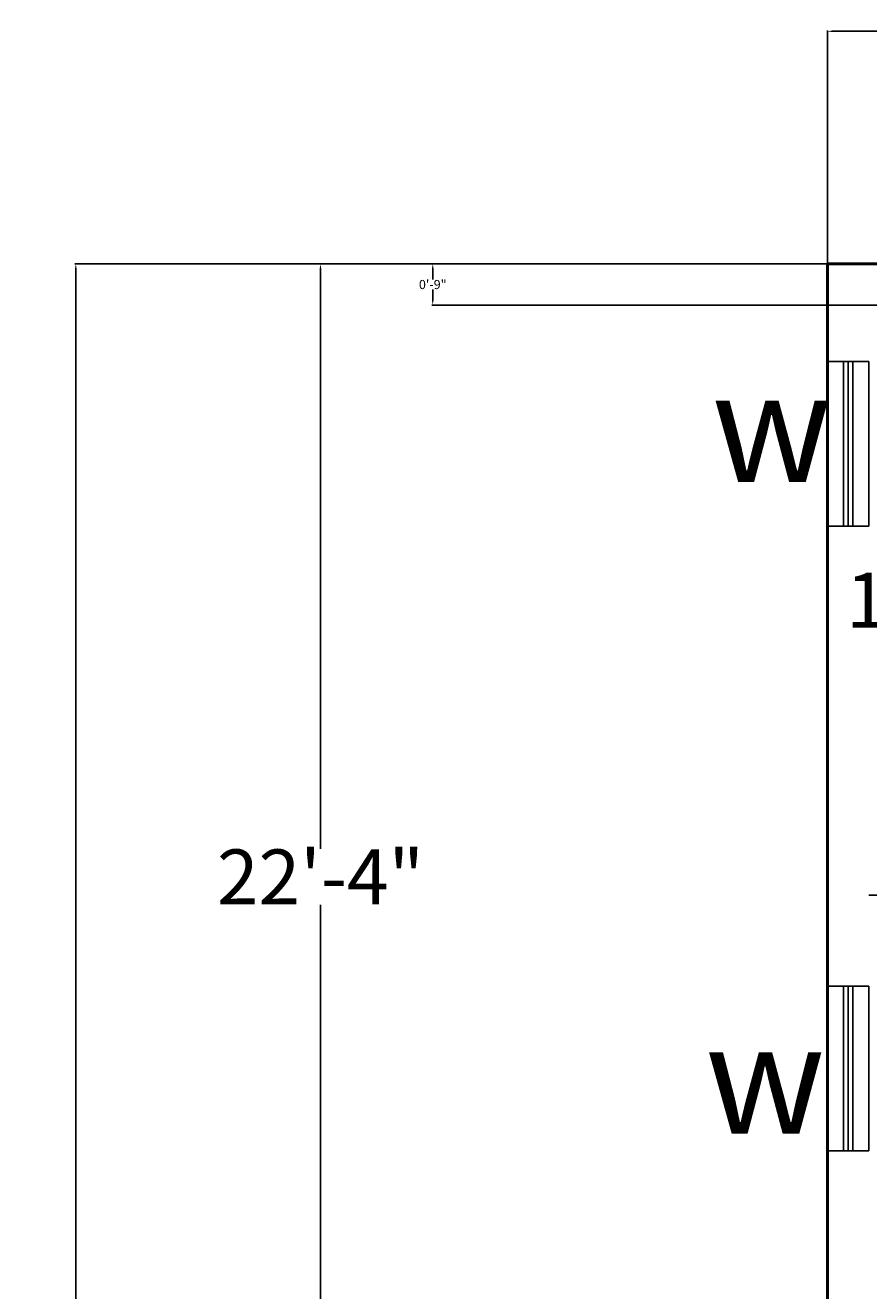
# Model space of a CAD drawing. Units: inches. Extents: x 409 to 7572, y 7 to 725.
# Tile 16 of 38: x 2800 to 2984, y 448 to 725. Entities that reach past the tile are written whole.
import ezdxf

# ---------------------------------------------------------------- set-up
doc = ezdxf.new("R2010")
doc.units = ezdxf.units.IN
doc.header["$MEASUREMENT"] = 0
for name, color, linetype, lineweight in [('A-ANNO-DIMS', 2, 'Continuous', 18), ('A-ANNO-SYMB', 3, 'Continuous', 25), ('A-GLAZ', 4, 'Continuous', 25), ('A-WALL', 7, 'Continuous', 50)]:
    doc.layers.add(name, color=color, linetype=linetype, lineweight=lineweight)
doc.styles.get("Standard").update_dxf_attribs({"font": 'arial.ttf'})
doc.dimstyles.get("Standard").update_dxf_attribs({"dimtxt": 2, "dimasz": 1, "dimexe": 0.18, "dimexo": 0.0625, "dimgap": 0.09, "dimtad": 0, "dimtih": 1, "dimtoh": 1, "dimdec": 0, "dimzin": 0, "dimdsep": 46, "dimlunit": 3, "dimtxsty": 'Standard', "dimcen": 0.09, "dimadec": 0, "dimazin": 0, "dimtfac": 1, "dimtdec": 0, "dimtofl": 0, "dimtmove": 0, "dimatfit": 3, "dimfxl": 1, "dimtolj": 1, "dimtzin": 0, "dimarcsym": 0})

# ---------------------------------------------------------------- blocks, each defined once
blk = doc.blocks.new('*D71')
at = {"layer": 'A-ANNO-DIMS', "color": 0, "lineweight": -2, "transparency": 16777216}
for p, q in [((2984.16, 663.53), (3001.93, 663.53)), ((3001.75, 662.53), (3001.75, 605.25)), ((3001.75, 535.53), (3001.75, 592.81)), ((2984.16, 534.53), (3001.93, 534.53))]:
    blk.add_line(p, q, dxfattribs=at)
at = {"layer": 'A-ANNO-DIMS', "color": 0, "transparency": 16777216}
for points in [[(3001.58, 662.53), (3001.92, 662.53), (3001.75, 663.53)], [(3001.58, 535.53), (3001.92, 535.53), (3001.75, 534.53)]]:
    blk.add_solid(points, dxfattribs=at)
at = {"layer": 'DEFPOINTS', "color": 0, "transparency": 16777216}
for p in [(2984.1, 663.53), (2984.1, 534.53), (3001.75, 534.53)]:
    blk.add_point(p, dxfattribs=at)
at = {"layer": 'A-ANNO-DIMS', "color": 0, "transparency": 16777216, "insert": (3001.75, 599.03), "char_height": 2, "attachment_point": 5}
blk.add_mtext('\\A1;{\\H6x;10\'-9"}', dxfattribs=at)
blk = doc.blocks.new('*D90')
at = {"layer": 'A-ANNO-DIMS', "color": 0, "lineweight": -2, "transparency": 16777216}
for p, q in [((2975.1, 672.59), (2975.1, 723.56)), ((2976.1, 723.38), (3242.53, 723.38)), ((3516.1, 723.38), (3249.66, 723.38)), ((3517.1, 672.59), (3517.1, 723.56))]:
    blk.add_line(p, q, dxfattribs=at)
at = {"layer": 'A-ANNO-DIMS', "color": 0, "transparency": 16777216}
for points in [[(2976.1, 723.55), (2976.1, 723.22), (2975.1, 723.38)], [(3516.1, 723.55), (3516.1, 723.22), (3517.1, 723.38)]]:
    blk.add_solid(points, dxfattribs=at)
at = {"layer": 'DEFPOINTS', "color": 0, "transparency": 16777216}
for p in [(2975.1, 723.38), (2975.1, 672.53), (3517.1, 672.53)]:
    blk.add_point(p, dxfattribs=at)
at = {"layer": 'A-ANNO-DIMS', "color": 0, "transparency": 16777216, "insert": (3246.1, 723.38), "char_height": 2, "attachment_point": 5}
blk.add_mtext('\\A1;45\'-2"', dxfattribs=at)
blk = doc.blocks.new('*D76')
at = {"layer": 'A-ANNO-DIMS', "color": 0, "lineweight": -2, "transparency": 16777216}
for p, q in [((2975.04, 672.53), (2864.14, 672.53)), ((2864.32, 671.53), (2864.32, 544.65)), ((2864.32, 405.53), (2864.32, 532.42)), ((2975.04, 404.53), (2864.14, 404.53))]:
    blk.add_line(p, q, dxfattribs=at)
at = {"layer": 'A-ANNO-DIMS', "color": 0, "transparency": 16777216}
for points in [[(2864.15, 671.53), (2864.48, 671.53), (2864.32, 672.53)], [(2864.15, 405.53), (2864.48, 405.53), (2864.32, 404.53)]]:
    blk.add_solid(points, dxfattribs=at)
at = {"layer": 'DEFPOINTS', "color": 0, "transparency": 16777216}
for p in [(2975.1, 672.53), (2864.32, 404.53), (2975.1, 404.53)]:
    blk.add_point(p, dxfattribs=at)
at = {"layer": 'A-ANNO-DIMS', "color": 0, "transparency": 16777216, "insert": (2864.32, 538.53), "char_height": 2, "attachment_point": 5}
blk.add_mtext('\\A1;{\\H6x;22\'-4"}', dxfattribs=at)
blk = doc.blocks.new('*D65')
at = {"layer": 'A-ANNO-DIMS', "color": 0, "lineweight": -2, "transparency": 16777216}
for p, q in [((2975.04, 672.53), (2810.68, 672.53)), ((2810.86, 671.53), (2810.86, 420.75)), ((2810.86, 157.53), (2810.86, 408.31)), ((2975.04, 156.53), (2810.68, 156.53))]:
    blk.add_line(p, q, dxfattribs=at)
at = {"layer": 'A-ANNO-DIMS', "color": 0, "transparency": 16777216}
for points in [[(2810.69, 671.53), (2811.03, 671.53), (2810.86, 672.53)], [(2810.69, 157.53), (2811.03, 157.53), (2810.86, 156.53)]]:
    blk.add_solid(points, dxfattribs=at)
at = {"layer": 'DEFPOINTS', "color": 0, "transparency": 16777216}
for p in [(2975.1, 672.53), (2810.86, 156.53), (2975.1, 156.53)]:
    blk.add_point(p, dxfattribs=at)
at = {"layer": 'A-ANNO-DIMS', "color": 0, "transparency": 16777216, "insert": (2810.86, 414.53), "char_height": 2, "attachment_point": 5}
blk.add_mtext("\\A1;{\\H6x;43'}", dxfattribs=at)
blk = doc.blocks.new('WIN-36')
for p, q in [((1699.82, 514.65), (1699.82, 478.65)), ((1700.82, 514.65), (1700.82, 478.65)), ((1701.82, 514.65), (1701.82, 478.65))]:
    blk.add_line(p, q)
blk.add_lwpolyline([(1705.32, 514.65), (1705.32, 478.65), (1696.32, 478.65), (1696.32, 514.65)], close=True)
blk = doc.blocks.new('*D183')
at = {"layer": 'A-ANNO-DIMS', "color": 0, "lineweight": -2, "transparency": 16777216}
for p, q in [((2975.04, 672.53), (2888.67, 672.53)), ((2888.85, 671.53), (2888.85, 669.14)), ((2888.85, 664.53), (2888.85, 666.92)), ((2984.04, 663.53), (2888.67, 663.53))]:
    blk.add_line(p, q, dxfattribs=at)
at = {"layer": 'A-ANNO-DIMS', "color": 0, "transparency": 16777216}
for points in [[(2888.68, 671.53), (2889.01, 671.53), (2888.85, 672.53)], [(2888.68, 664.53), (2889.01, 664.53), (2888.85, 663.53)]]:
    blk.add_solid(points, dxfattribs=at)
at = {"layer": 'DEFPOINTS', "color": 0, "transparency": 16777216}
for p in [(2975.1, 672.53), (2888.85, 663.53), (2984.1, 663.53)]:
    blk.add_point(p, dxfattribs=at)
at = {"layer": 'A-ANNO-DIMS', "color": 0, "transparency": 16777216, "insert": (2888.85, 668.03), "char_height": 2, "attachment_point": 5}
blk.add_mtext('\\A1;0\'-9"', dxfattribs=at)

msp = doc.modelspace()

# ---------------------------------------------------------------- linework, layer by layer
at = {"layer": 'A-WALL'}
for p, q in [((3517.1, 672.53), (2975.1, 672.53)), ((2975.1, 672.53), (2975.1, 404.53))]:
    msp.add_line(p, q, dxfattribs=at)

# ---------------------------------------------------------------- block references
at = {"layer": 'A-GLAZ'}
for p in [(1278.78, 136.58), (1278.78, 0)]:
    msp.add_blockref('WIN-36', p, dxfattribs=at)

# ---------------------------------------------------------------- texts
at = {"layer": 'A-ANNO-SYMB', "char_height": 24, "attachment_point": 1}
for insert in [(2949.76, 648.83), (2948.34, 506.39)]:
    msp.add_mtext_dynamic_manual_height_columns('w', width=18.2582, gutter_width=1, heights=[0], dxfattribs=dict(at, insert=insert))

# ---------------------------------------------------------------- dimensions: what is measured, and where the dimension line sits
at = {"layer": 'A-ANNO-DIMS'}
dim = msp.add_linear_dim(base=(2975.1, 723.38), p1=(3517.1, 672.53), p2=(2975.1, 672.53), dimstyle='Standard', override={"dimclrd": 0, "dimclre": 0, "dimclrt": 0}, dxfattribs=at)
dim.commit()
dim.dimension.update_dxf_attribs({"geometry": '*D90', "text_midpoint": (3246.1, 723.38)})
for base, p1, p2, picture, middle in [((2810.86, 156.53), (2975.1, 672.53), (2975.1, 156.53), '*D65', (2810.86, 414.53)), ((2864.32, 404.53), (2975.1, 672.53), (2975.1, 404.53), '*D76', (2864.32, 538.53)), ((3001.75, 534.53), (2984.1, 663.53), (2984.1, 534.53), '*D71', (3001.75, 599.03))]:
    dim = msp.add_linear_dim(base=base, p1=p1, p2=p2, angle=90, text='{\\H6x;<>}', dimstyle='Standard', override={"dimclrd": 0, "dimclre": 0, "dimclrt": 0}, dxfattribs=at)
    dim.commit()
    dim.dimension.update_dxf_attribs({"geometry": picture, "text_midpoint": middle})
dim = msp.add_linear_dim(base=(2888.85, 663.53), p1=(2975.1, 672.53), p2=(2984.1, 663.53), angle=90, dimstyle='Standard', override={"dimdec": 1, "dimlfac": 1, "dimrnd": 0, "dimzin": 1, "dimdsep": 46, "dimlunit": 4, "dimfrac": 2}, dxfattribs=at)
dim.commit()
dim.dimension.update_dxf_attribs({"geometry": '*D183', "text_midpoint": (2888.85, 668.03)})

doc.saveas('drawing.dxf')
